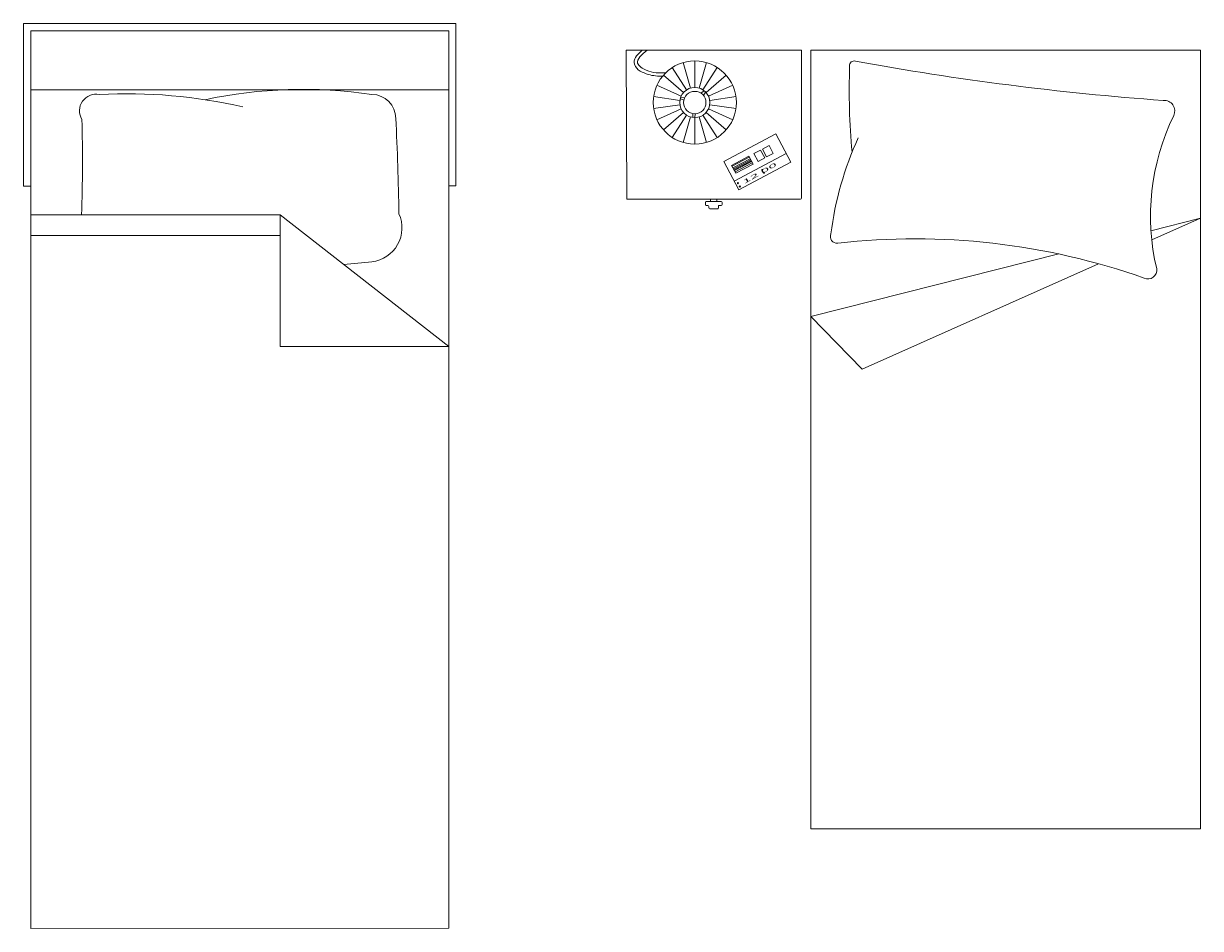
# Model space of a CAD drawing. Units: inches. Extents: x 1994 to 3075, y 3517 to 3950.
# Tile 14 of 58: x 1994.4081 to 1994.5301, y 3553.3477 to 3553.4416. Entities that reach past the tile are written whole.
import ezdxf

# ---------------------------------------------------------------- set-up
doc = ezdxf.new("R2010")
doc.units = ezdxf.units.IN
doc.layers.add('A-FURN-REFR', color=8, linetype='Continuous', lineweight=13)
doc.layers.add('A-FURN-REFR-TEXT', color=7, linetype='Continuous', lineweight=13)
doc.styles.get("Standard").update_dxf_attribs({"font": 'arial.ttf'})

msp = doc.modelspace()

# ---------------------------------------------------------------- linework, layer by layer
at = {"layer": 'A-FURN-REFR'}
for p, q in [((1994.408098659575, 3553.424699404811), (1994.408098659575, 3553.441574404811)), ((1994.408098659575, 3553.441574404811), (1994.452927590283, 3553.441574404811)), ((1994.408848659575, 3553.440824404811), (1994.452177590283, 3553.440824404811)), ((1994.408848659575, 3553.440824404811), (1994.408848659575, 3553.424699404811)), ((1994.452177590283, 3553.440824404811), (1994.452177590283, 3553.347733986448)), ((1994.452927590283, 3553.424734016448), (1994.452927590283, 3553.441574404811)), ((1994.488740066537, 3553.438811118921), (1994.470566855357, 3553.438811118921)), ((1994.488740066537, 3553.438811118921), (1994.470566855357, 3553.438811118921)), ((1994.470661360515, 3553.423366487403), (1994.470566855357, 3553.438811118921)), ((1994.488740066537, 3553.438811118921), (1994.488740066537, 3553.423460992562)), ((1994.489733353897, 3553.438811118921), (1994.530118267633, 3553.438811118921)), ((1994.489733353897, 3553.423366487403), (1994.489733353897, 3553.438811118921)), ((1994.489733353897, 3553.438811118921), (1994.530118267633, 3553.438811118921)), ((1994.530118267633, 3553.438811118921), (1994.530118267633, 3553.358041291449)), ((1994.530118267633, 3553.438811118921), (1994.530118267633, 3553.358041291449)), ((1994.475360326966, 3553.43701005636), (1994.476848666523, 3553.434694154804)), ((1994.476477879105, 3553.437520425322), (1994.477253465586, 3553.434879020341)), ((1994.477693950083, 3553.437695269932), (1994.477693950083, 3553.434942352451)), ((1994.477693950083, 3553.437695269932), (1994.477693950083, 3553.434942352451)), ((1994.47891002106, 3553.437520425322), (1994.47813443458, 3553.434879020341)), ((1994.478539233642, 3553.434694154804), (1994.480027573199, 3553.43701005636)), ((1994.474431831093, 3553.436205510107), (1994.476512347308, 3553.434402732545)), ((1994.478875552857, 3553.434402732545), (1994.480956069072, 3553.436205510107)), ((1994.408848659575, 3553.347699374811), (1994.408848659575, 3553.434699404812)), ((1994.408848659575, 3553.434699404812), (1994.452177590283, 3553.434699404812)), ((1994.4737676127, 3553.435171966113), (1994.476271754522, 3553.434028362862)), ((1994.47830597362, 3553.43436247168), (1994.478663599735, 3553.434605352097)), ((1994.478588575116, 3553.43411486739), (1994.478812825867, 3553.434470930586)), ((1994.479116145644, 3553.434028362862), (1994.481620287465, 3553.435171966113)), ((1994.473421482812, 3553.433993155967), (1994.476146379562, 3553.433601374962)), ((1994.473421482812, 3553.432764579856), (1994.476146379562, 3553.433156360862)), ((1994.476562602356, 3553.433628069643), (1994.476186634651, 3553.433794179955)), ((1994.476641731474, 3553.433863517456), (1994.476231502336, 3553.433931796923)), ((1994.479241520604, 3553.433601374962), (1994.481966417354, 3553.433993155967)), ((1994.479241520604, 3553.433156360862), (1994.481966417354, 3553.432764579856)), ((1994.4737676127, 3553.431585769711), (1994.476271754522, 3553.432729372962)), ((1994.474431831093, 3553.430552225717), (1994.476512347308, 3553.43235500328)), ((1994.475360326966, 3553.429747679464), (1994.476848666523, 3553.43206358102)), ((1994.477253465586, 3553.431878715482), (1994.476477879105, 3553.429237310503)), ((1994.477483387212, 3553.432239696082), (1994.477486235193, 3553.431829242658)), ((1994.477751671973, 3553.432221838369), (1994.47764967673, 3553.431816010345)), ((1994.47813443458, 3553.431878715482), (1994.47891002106, 3553.429237310503)), ((1994.478539233642, 3553.43206358102), (1994.480027573199, 3553.429747679464)), ((1994.478875552857, 3553.43235500328), (1994.480956069072, 3553.430552225717)), ((1994.479116145644, 3553.432729372962), (1994.481620287465, 3553.431585769711)), ((1994.477693950083, 3553.431815383373), (1994.477693950083, 3553.429062465891)), ((1994.477693950083, 3553.431815383373), (1994.477693950083, 3553.429062465891)), ((1994.486102364336, 3553.430117008454), (1994.480693358694, 3553.427249603569)), ((1994.487656993033, 3553.427184393169), (1994.486102364336, 3553.430117008454)), ((1994.48450803375, 3553.428450938641), (1994.483824100177, 3553.428088373948)), ((1994.484945645817, 3553.427625437453), (1994.48450803375, 3553.428450938641)), ((1994.48538850957, 3553.428917693685), (1994.484704575997, 3553.428555128993)), ((1994.484704575997, 3553.428555128993), (1994.485142188064, 3553.427729627804)), ((1994.485826121637, 3553.428092192496), (1994.48538850957, 3553.428917693685)), ((1994.480693358694, 3553.427249603569), (1994.482247987391, 3553.424316988284)), ((1994.481506919476, 3553.426859997478), (1994.483292763387, 3553.427806703377)), ((1994.481558750892, 3553.426762223903), (1994.483344594803, 3553.427708929803)), ((1994.481641878191, 3553.426605414507), (1994.483427722103, 3553.427552120407)), ((1994.481701163511, 3553.426493580063), (1994.483487007423, 3553.427440285963)), ((1994.481753146848, 3553.426395519912), (1994.483538990759, 3553.427342225811)), ((1994.487172371131, 3553.428098572613), (1994.481763365488, 3553.425231167728)), ((1994.481797827318, 3553.426311235715), (1994.483583671229, 3553.427257941616)), ((1994.481868283148, 3553.426178329482), (1994.483654127059, 3553.427125035381)), ((1994.481944531543, 3553.426034496289), (1994.483730375454, 3553.426981202189)), ((1994.482247987391, 3553.424316988284), (1994.487656993033, 3553.427184393169)), ((1994.483730375454, 3553.426981202189), (1994.483292763387, 3553.427806703377)), ((1994.483824100177, 3553.428088373948), (1994.484261712244, 3553.42726287276)), ((1994.484261712244, 3553.42726287276), (1994.484945645817, 3553.427625437453)), ((1994.485142188064, 3553.427729627804), (1994.485826121637, 3553.428092192496)), ((1994.481506919476, 3553.426859997478), (1994.481944531543, 3553.426034496289)), ((1994.408848659575, 3553.424699404811), (1994.408098659575, 3553.424699404811)), ((1994.452927590283, 3553.424734016448), (1994.452177590283, 3553.424734016448)), ((1994.470661360515, 3553.423366487403), (1994.488645561379, 3553.423366487403)), ((1994.47997236635, 3553.423366487403), (1994.479334555544, 3553.423366487403)), ((1994.479334555544, 3553.423366487403), (1994.479334555544, 3553.42309596792)), ((1994.47997236635, 3553.42309596792), (1994.47997236635, 3553.423366487403)), ((1994.489733353897, 3553.358041291449), (1994.489733353897, 3553.423366487403)), ((1994.489733353897, 3553.358041291449), (1994.489733353897, 3553.423366487403)), ((1994.47879173547, 3553.423001462762), (1994.47879173547, 3553.422790853514)), ((1994.480420681265, 3553.42309596792), (1994.478886240629, 3553.42309596792)), ((1994.478886240629, 3553.422696348356), (1994.479053799294, 3553.422696348356)), ((1994.479148304452, 3553.422601843198), (1994.479148304452, 3553.422444587389)), ((1994.47924280961, 3553.422350082231), (1994.480064112284, 3553.422350082231)), ((1994.480158617442, 3553.422444587389), (1994.480158617442, 3553.422696348356)), ((1994.480158617442, 3553.422696348356), (1994.480420681265, 3553.422696348356)), ((1994.480515186424, 3553.422790853514), (1994.480515186424, 3553.423001462762)), ((1994.408849859575, 3553.421739404811), (1994.434715159576, 3553.421739404811)), ((1994.434715159576, 3553.421739404811), (1994.434715159576, 3553.408059404811)), ((1994.452177590283, 3553.408059404811), (1994.434715159576, 3553.421739404811)), ((1994.530118267633, 3553.421377539334), (1994.524987428819, 3553.420082608042)), ((1994.530118267633, 3553.421377539334), (1994.525068414873, 3553.41912265896)), ((1994.434715159576, 3553.419579404811), (1994.408849859575, 3553.419579404811)), ((1994.515426041207, 3553.417669486044), (1994.489722498641, 3553.411182374916)), ((1994.519547030833, 3553.416657228561), (1994.495053945405, 3553.405720478471)), ((1994.495053945405, 3553.405720478471), (1994.489733353897, 3553.411185114587)), ((1994.434715159576, 3553.408059404811), (1994.452177590283, 3553.408059404811)), ((1994.530118267633, 3553.358041291449), (1994.489733353897, 3553.358041291449)), ((1994.530118267633, 3553.358041291449), (1994.489733353897, 3553.358041291449)), ((1994.452177590283, 3553.347733986448), (1994.408848659575, 3553.347699374811))]:
    msp.add_line(p, q, dxfattribs=at)
for radius in [0.0043164020201009, 0.0015634845390022, 0.0011584684638608]:
    msp.add_circle((1994.477693950083, 3553.433378867912), radius, dxfattribs=at)
for centre, radius, start, end in [((1994.562637066447, 3553.434620891056), 0.0689357559366832, 177.8833686819633, 185.3330513938759), ((1994.494190036177, 3553.437243584038), 0.0004482907065646, 70.44410133489674, 189.842981094497), ((1994.548148519904, 3553.732410615152), 0.2996159645214514, 259.654043260426, 265.8105338606814), ((1994.4188115066, 3553.380653114887), 0.0536356196908511, 77.05638185161688, 93.04883220562752), ((1994.4188115066, 3553.380653114887), 0.0536356196908511, 77.05638185161688, 93.04883220562752), ((1994.437047056808, 3553.386421743276), 0.0483256070365364, 81.47022635647696, 102.1032641982298), ((1994.437047056808, 3553.386421743276), 0.0483256070365364, 81.47022635647696, 102.1032641982298), ((1994.415622236877, 3553.432524291301), 0.0017217387327707, 78.72778623498706, 211.6094986857782), ((1994.415622236877, 3553.432524291301), 0.0017217387327707, 78.72778623498706, 211.6094986857782), ((1994.444214871835, 3553.431735233351), 0.0024775836026722, 0, 90), ((1994.444214871835, 3553.431735233351), 0.0024775836026722, 0, 90), ((1994.526356258471, 3553.432500927302), 0.0010985341214448, 334.0063374253624, 95.02047578612859), ((1994.548711344171, 3553.421600684199), 0.0237724360313189, 154.0063374253624, 193.3195713203381), ((1994.236830708058, 3553.427276528461), 0.1773784605747312, 358.2111392619709, 1.403751564921032), ((1994.236830708058, 3553.427276528461), 0.1773784605747312, 358.2111392619709, 1.403751564921032), ((1994.152000222532, 3553.417146749838), 0.2950531070603349, 0.9125644663952034, 2.834064295864955), ((1994.152000222532, 3553.417146749838), 0.2950531070603349, 0.9125644663952034, 2.834064295864955), ((1994.526739365545, 3553.41517084859), 0.0352435291682938, 155.6022979544526, 172.5426679115163), ((1994.48468690211, 3553.426382237387), 5.53897148363e-05, 90, 270), ((1994.48468690211, 3553.426382237387), 5.53897148363e-05, 270, 90), ((1994.484859017059, 3553.426102322342), 5.53897148363e-05, 90, 270), ((1994.484859017059, 3553.426102322342), 5.53897148363e-05, 270, 90), ((1994.482161557148, 3553.425014430974), 5.53897148363e-05, 90, 270), ((1994.482161557148, 3553.425014430974), 5.53897148363e-05, 270, 90), ((1994.482361684866, 3553.42466483445), 5.53897148363e-05, 90, 270), ((1994.482361684866, 3553.42466483445), 5.53897148363e-05, 270, 90), ((1994.488645561379, 3553.423460992562), 9.45051583805e-05, 270, 0), ((1994.478886240629, 3553.423001462762), 9.45051583805e-05, 90, 180), ((1994.478886240629, 3553.422790853514), 9.45051583805e-05, 180, 270), ((1994.479053799294, 3553.422601843198), 9.45051583805e-05, 0, 90), ((1994.47924280961, 3553.422444587389), 9.45051583805e-05, 180, 270), ((1994.480064112284, 3553.422444587389), 9.45051583805e-05, 270, 0), ((1994.480420681265, 3553.423001462762), 9.45051583805e-05, 0, 90), ((1994.480420681265, 3553.422790853514), 9.45051583805e-05, 270, 0), ((1994.443781134166, 3553.420380323964), 0.0035513056944607, 277.015318444972, 24.37436785420747), ((1994.443781134166, 3553.420380323964), 0.0035513056944607, 277.015318444972, 24.37436785420747), ((1994.492428897005, 3553.419480141639), 0.0006880002040652, 157.3555290337801, 276.462021683575), ((1994.5005163872, 3553.348076382541), 0.0711723108928986, 70.4847636335054, 96.46202168357497), ((1994.429816021691, 3553.554141992109), 0.1380394109326758, 274.7720352878431, 275.9873971424126), ((1994.429816021691, 3553.554141992109), 0.1380394109326758, 274.7720352878431, 275.9873971424126), ((1994.524677002065, 3553.41598656695), 0.0009117868872928, 245.0255496401715, 8.665342121911433)]:
    msp.add_arc(centre, radius, start, end, dxfattribs=at)
for points, knots in [([(1994.474356308012, 3553.43611592323), (1994.473884058442, 3553.436112073895), (1994.473382821048, 3553.436132341107), (1994.472316171806, 3553.436465510121), (1994.471644088965, 3553.436717237969), (1994.471282314951, 3553.437871796533), (1994.471682284241, 3553.438292070641), (1994.472127903637, 3553.438699949725), (1994.472191495253, 3553.438755806477), (1994.472256010091, 3553.438811118921)], [0.0077183477163671, 0.0077183477163671, 0.0077183477163671, 0.0077183477163671, 0.0428867239757183, 0.0428867239757183, 0.0785443346356031, 0.0785443346356031, 0.1084777623087474, 0.1084777623087474, 0.1132872864949097, 0.1132872864949097, 0.1132872864949097, 0.1132872864949097]), ([(1994.474656950513, 3553.436446107715), (1994.474003701164, 3553.436433875138), (1994.472981229165, 3553.436427038187), (1994.471254074305, 3553.437551565143), (1994.472197765358, 3553.438343482311), (1994.472763214703, 3553.438811118921)], [0, 0, 0, 0, 0.0020194675198324, 0.0031659294013677, 0.0048546887776152, 0.0048546887776152, 0.0048546887776152, 0.0048546887776152])]:
    msp.add_open_spline(points, degree=3, knots=knots, dxfattribs=at)

# ---------------------------------------------------------------- texts
at = {"layer": 'A-FURN-REFR-TEXT', "width": 3}
msp.add_text('12 00', height=0.000395772154613, rotation=29.3564842939468, dxfattribs=at).set_placement((1994.482790599524, 3553.424909755842))

doc.saveas('drawing.dxf')
